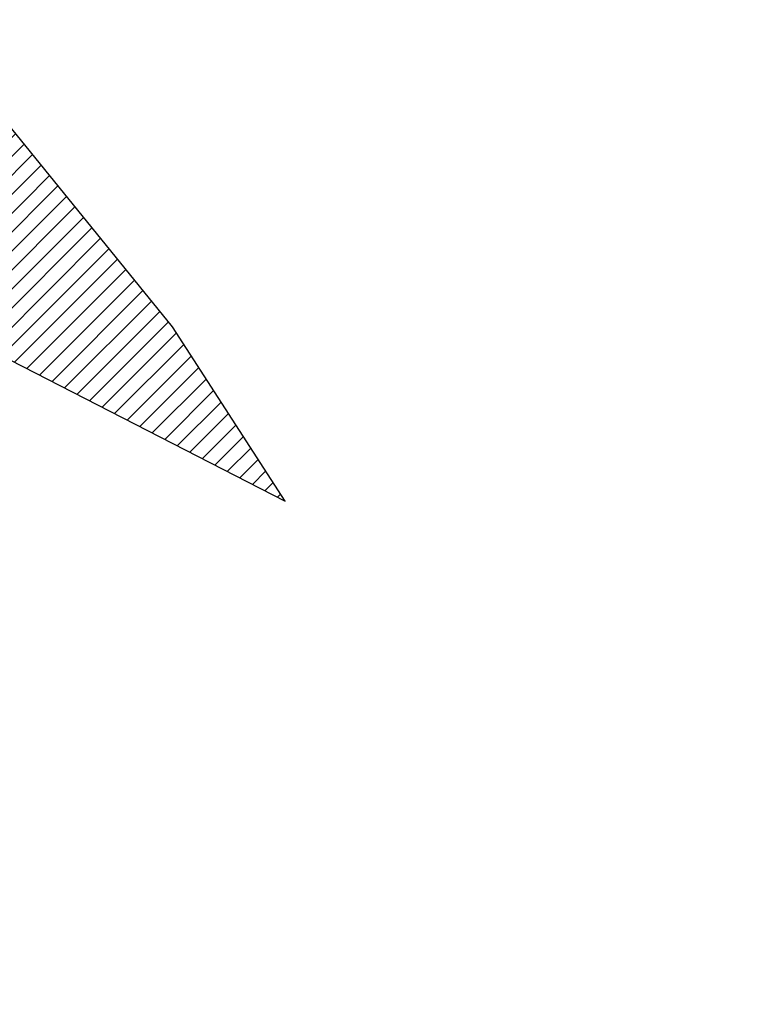
# Model space of a CAD drawing. Units: inches. Extents: x 1986 to 21484, y -1816 to 2016.
# Tile 28 of 85: x 2182.45 to 2190.96, y 1865.09 to 1876.39. Entities that reach past the tile are written whole.
import ezdxf

# ---------------------------------------------------------------- set-up
doc = ezdxf.new("R2010")
doc.units = ezdxf.units.IN
doc.layers.add('L-PLNT', color=84, linetype='Continuous', lineweight=13)
doc.layers.add('vfolhas', color=114, linetype='Continuous', lineweight=5)
doc.layers.add('vfolha', color=72, linetype='Continuous')

# ---------------------------------------------------------------- blocks, each defined once
blk = doc.blocks.new('arbusto_PB_verde_grande')
at = {"layer": 'vfolhas'}
h = blk.add_hatch(dxfattribs=at)
h.set_pattern_fill('ANSI31', color=256, scale=0.05, style=0)
h.set_pattern_definition([(45, (-2446.5133113, 50.986076), (-0.004419417382, 0.004419417382), [])])
h.paths.add_polyline_path([(-0.07279, 0.50669), (-0.18085, 0.65063), (-0.2334, 0.67253), (-0.20712, 0.53176), (-0.10785, 0.25007), (0.02625, -0.03934), (0.00028, 0.09048), (0.00816, 0.16241), (-0.04939, 0.29079)])
h.paths.add_polyline_path([(0.09902, 0.41929), (0.09372, 0.26573), (0.07906, 0.18814), (0.15506, 0.36901), (0.26606, 0.5505), (0.28356, 0.63504), (0.2485, 0.68819), (0.25145, 0.63504), (0.20178, 0.54426)])
h.paths.add_polyline_path([(0.12295, 0.24073), (0.047, 0.06233), (0.02625, -0.03934), (0.11122, 0.04358), (0.18428, 0.09364), (0.27478, 0.19376), (0.3215, 0.25323), (0.44129, 0.38467), (0.47634, 0.57866), (0.41789, 0.45347), (0.28939, 0.30954)])
h.paths.add_polyline_path([(0.58145, -0.03779), (0.70707, 0.01536), (0.78591, 0.04667), (0.74796, 0.06549), (0.62818, 0.08423), (0.52595, 0.09048), (0.39745, 0.04358), (0.02625, -0.03934), (0.25728, -0.03154), (0.43834, -0.0347)])
h.paths.add_polyline_path([(0.52022, -0.03647), (0.43834, -0.0347), (0.25728, -0.03154), (0.02625, -0.03934), (0.17964, -0.08515), (0.53768, -0.13167), (0.69541, -0.15357), (0.78591, -0.07852), (0.70413, -0.10042)])
h.paths.add_polyline_path([(0.27189, -0.21929), (0.14922, -0.14107), (0.02625, -0.03934), (0.15794, -0.31007), (0.29522, -0.42585), (0.41789, -0.49157), (0.56396, -0.56669), (0.5114, -0.48532), (0.39456, -0.34139)])
h.paths.add_polyline_path([(-0.05818, -0.47591), (-0.02312, -0.61984), (0.047, -0.80134), (0.08494, -0.59794), (0.07911, -0.4071), (0.03527, -0.25376), (0.02625, -0.03934), (-0.03773, -0.26001)])
h.paths.add_polyline_path([(-0.24218, 0.14054), (-0.11073, 0.06858), (0.02625, -0.03934), (-0.04235, 0.10871), (-0.21007, 0.23757), (-0.36485, 0.33145), (-0.47874, 0.40341), (-0.54303, 0.46288), (-0.49041, 0.33145), (-0.39408, 0.22192)])
at = {"layer": 'vfolha'}
for p, q in [((0.5114, -0.48532), (0.39456, -0.34139)), ((0.56396, -0.56669), (0.5114, -0.48532)), ((0.41789, -0.49157), (0.56396, -0.56669))]:
    blk.add_line(p, q, dxfattribs=at)

msp = doc.modelspace()

# ---------------------------------------------------------------- block references
at = {"layer": 'L-PLNT', "xscale": 24.60366729364114, "yscale": 24.60366729364114, "zscale": 24.60366729364114}
msp.add_blockref('arbusto_PB_verde_grande', (2171.623, 1884.805), dxfattribs=at)

doc.saveas('drawing.dxf')
